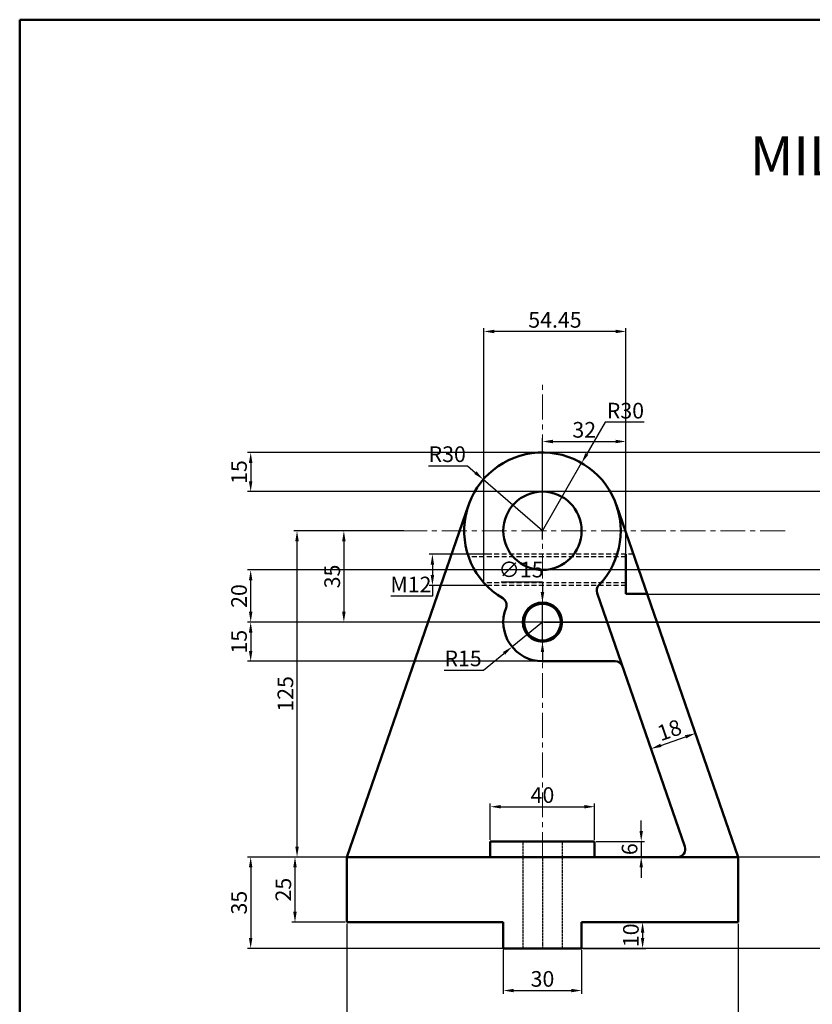
# Model space of a CAD drawing. Units: millimetres. Extents: x 177 to 1064, y 105 to 671.
# Tile 2 of 4: x 177 to 480, y 294 to 671. Entities that reach past the tile are written whole.
import ezdxf

# ---------------------------------------------------------------- set-up
doc = ezdxf.new("R2010")
doc.units = ezdxf.units.MM
doc.header["$LTSCALE"] = 0.3
doc.linetypes.add('CENTER', pattern=[50.8, 31.75, -6.35, 6.35, -6.35])
doc.linetypes.add('HIDDEN', pattern=[9.525, 6.35, -3.175])
for name, color, linetype, lineweight in [('M-CNTR', 1, 'CENTER', 18), ('M-DIMS', 2, 'Continuous', 25), ('M-HIDN', 6, 'HIDDEN', 25), ('M-OUTL', 7, 'Continuous', 50), ('M-TEXT', 3, 'Continuous', 25)]:
    doc.layers.add(name, color=color, linetype=linetype, lineweight=lineweight)
doc.styles.get("Standard").update_dxf_attribs({"font": 'arial.ttf'})
doc.dimstyles.new('ISO-25', dxfattribs={"dimtxt": 6, "dimasz": 4, "dimexe": 1.25, "dimexo": 0.625, "dimtad": 1, "dimtoh": 1, "dimtxsty": 'Standard', "dimcen": 2.5, "dimadec": 0, "dimazin": 0, "dimtfac": 1, "dimtmove": 0, "dimatfit": 3, "dimfxl": 1, "dimarcsym": 0})

# ---------------------------------------------------------------- blocks, each defined once
blk = doc.blocks.new('*D1')
at = {"layer": 'Defpoints', "color": 0, "ltscale": 0.2, "transparency": 16777216}
for p in [(302.04, 325.34), (452.04, 325.34), (452.04, 278.47)]:
    blk.add_point(p, dxfattribs=at)
at = {"layer": 'M-DIMS', "color": 0, "lineweight": -2, "ltscale": 0.2, "transparency": 16777216}
for p, q in [((302.04, 324.72), (302.04, 277.22)), ((452.04, 324.72), (452.04, 277.22)), ((306.04, 278.47), (448.04, 278.47))]:
    blk.add_line(p, q, dxfattribs=at)
at = {"layer": 'M-DIMS', "color": 0, "ltscale": 0.2, "transparency": 16777216}
for points in [[(306.04, 279.14), (306.04, 277.81), (302.04, 278.47)], [(448.04, 279.14), (448.04, 277.81), (452.04, 278.47)]]:
    blk.add_solid(points, dxfattribs=at)
at = {"layer": 'M-DIMS', "color": 0, "ltscale": 0.2, "transparency": 16777216, "insert": (377.04, 282.16), "char_height": 6, "attachment_point": 5}
blk.add_mtext('150', dxfattribs=at)
blk = doc.blocks.new('*D2')
at = {"layer": 'Defpoints', "color": 0, "ltscale": 0.2, "transparency": 16777216}
for p in [(362.04, 315.34), (392.04, 315.34), (392.04, 299.16)]:
    blk.add_point(p, dxfattribs=at)
at = {"layer": 'M-DIMS', "color": 0, "lineweight": -2, "ltscale": 0.2, "transparency": 16777216}
for p, q in [((362.04, 314.72), (362.04, 297.91)), ((392.04, 314.72), (392.04, 297.91)), ((366.04, 299.16), (388.04, 299.16))]:
    blk.add_line(p, q, dxfattribs=at)
at = {"layer": 'M-DIMS', "color": 0, "ltscale": 0.2, "transparency": 16777216}
for points in [[(366.04, 299.83), (366.04, 298.5), (362.04, 299.16)], [(388.04, 299.83), (388.04, 298.5), (392.04, 299.16)]]:
    blk.add_solid(points, dxfattribs=at)
at = {"layer": 'M-DIMS', "color": 0, "ltscale": 0.2, "transparency": 16777216, "insert": (377.04, 302.85), "char_height": 6, "attachment_point": 5}
blk.add_mtext('30', dxfattribs=at)
blk = doc.blocks.new('*D3')
at = {"layer": 'Defpoints', "color": 0, "ltscale": 0.2, "transparency": 16777216}
for p in [(302.04, 350.34), (282.23, 325.34), (302.04, 325.34)]:
    blk.add_point(p, dxfattribs=at)
at = {"layer": 'M-DIMS', "color": 0, "lineweight": -2, "ltscale": 0.2, "transparency": 16777216}
for p, q in [((301.42, 350.34), (280.98, 350.34)), ((282.23, 346.34), (282.23, 329.34)), ((301.42, 325.34), (280.98, 325.34))]:
    blk.add_line(p, q, dxfattribs=at)
at = {"layer": 'M-DIMS', "color": 0, "ltscale": 0.2, "transparency": 16777216}
for points in [[(281.56, 346.34), (282.89, 346.34), (282.23, 350.34)], [(281.56, 329.34), (282.89, 329.34), (282.23, 325.34)]]:
    blk.add_solid(points, dxfattribs=at)
at = {"layer": 'M-DIMS', "color": 0, "ltscale": 0.2, "transparency": 16777216, "insert": (278.54, 337.84), "char_height": 6, "attachment_point": 5, "rotation": 90}
blk.add_mtext('25', dxfattribs=at)
blk = doc.blocks.new('*D4')
at = {"layer": 'Defpoints', "color": 0, "ltscale": 0.2, "transparency": 16777216}
for p in [(283.01, 475.34), (302.04, 475.34), (302.04, 350.34)]:
    blk.add_point(p, dxfattribs=at)
at = {"layer": 'M-DIMS', "color": 0, "lineweight": -2, "ltscale": 0.2, "transparency": 16777216}
for p, q in [((301.42, 475.34), (281.76, 475.34)), ((283.01, 354.34), (283.01, 471.34)), ((301.42, 350.34), (281.76, 350.34))]:
    blk.add_line(p, q, dxfattribs=at)
at = {"layer": 'M-DIMS', "color": 0, "ltscale": 0.2, "transparency": 16777216}
for points in [[(282.35, 471.34), (283.68, 471.34), (283.01, 475.34)], [(282.35, 354.34), (283.68, 354.34), (283.01, 350.34)]]:
    blk.add_solid(points, dxfattribs=at)
at = {"layer": 'M-DIMS', "color": 0, "ltscale": 0.2, "transparency": 16777216, "insert": (279.33, 412.84), "char_height": 6, "attachment_point": 5, "rotation": 90}
blk.add_mtext('125', dxfattribs=at)
blk = doc.blocks.new('*D5')
at = {"layer": 'Defpoints', "color": 0, "ltscale": 0.2, "transparency": 16777216}
for p in [(397.04, 369.61), (357.04, 356.34), (397.04, 356.34)]:
    blk.add_point(p, dxfattribs=at)
at = {"layer": 'M-DIMS', "color": 0, "lineweight": -2, "ltscale": 0.2, "transparency": 16777216}
for p, q in [((357.04, 356.97), (357.04, 370.86)), ((397.04, 356.97), (397.04, 370.86)), ((361.04, 369.61), (393.04, 369.61))]:
    blk.add_line(p, q, dxfattribs=at)
at = {"layer": 'M-DIMS', "color": 0, "ltscale": 0.2, "transparency": 16777216}
for points in [[(361.04, 370.28), (361.04, 368.94), (357.04, 369.61)], [(393.04, 370.28), (393.04, 368.94), (397.04, 369.61)]]:
    blk.add_solid(points, dxfattribs=at)
at = {"layer": 'M-DIMS', "color": 0, "ltscale": 0.2, "transparency": 16777216, "insert": (377.04, 373.3), "char_height": 6, "attachment_point": 5}
blk.add_mtext('40', dxfattribs=at)
blk = doc.blocks.new('*D6')
at = {"layer": 'Defpoints', "color": 0, "ltscale": 0.2, "transparency": 16777216}
for p in [(397.04, 356.34), (397.04, 350.34), (414.87, 350.34)]:
    blk.add_point(p, dxfattribs=at)
at = {"layer": 'M-DIMS', "color": 0, "lineweight": -2, "ltscale": 0.2, "transparency": 16777216}
for p, q in [((414.87, 360.34), (414.87, 364.34)), ((397.67, 356.34), (416.12, 356.34)), ((414.87, 356.34), (414.87, 350.34)), ((397.67, 350.34), (416.12, 350.34)), ((414.87, 346.34), (414.87, 342.34))]:
    blk.add_line(p, q, dxfattribs=at)
at = {"layer": 'M-DIMS', "color": 0, "ltscale": 0.2, "transparency": 16777216}
for points in [[(414.21, 360.34), (415.54, 360.34), (414.87, 356.34)], [(414.21, 346.34), (415.54, 346.34), (414.87, 350.34)]]:
    blk.add_solid(points, dxfattribs=at)
at = {"layer": 'M-DIMS', "color": 0, "ltscale": 0.2, "transparency": 16777216, "insert": (411.19, 353.34), "char_height": 6, "attachment_point": 5, "rotation": 90}
blk.add_mtext('6', dxfattribs=at)
blk = doc.blocks.new('*D7')
at = {"layer": 'Defpoints', "color": 0, "ltscale": 0.2, "transparency": 16777216}
for p in [(392.04, 325.34), (392.04, 315.34), (415.4, 315.34)]:
    blk.add_point(p, dxfattribs=at)
at = {"layer": 'M-DIMS', "color": 0, "lineweight": -2, "ltscale": 0.2, "transparency": 16777216}
for p, q in [((392.67, 325.34), (416.65, 325.34)), ((415.4, 321.34), (415.4, 319.34)), ((392.67, 315.34), (416.65, 315.34))]:
    blk.add_line(p, q, dxfattribs=at)
at = {"layer": 'M-DIMS', "color": 0, "ltscale": 0.2, "transparency": 16777216}
for points in [[(414.74, 321.34), (416.07, 321.34), (415.4, 325.34)], [(414.74, 319.34), (416.07, 319.34), (415.4, 315.34)]]:
    blk.add_solid(points, dxfattribs=at)
at = {"layer": 'M-DIMS', "color": 0, "ltscale": 0.2, "transparency": 16777216, "insert": (411.71, 320.34), "char_height": 6, "attachment_point": 5, "rotation": 90}
blk.add_mtext('10', dxfattribs=at)
blk = doc.blocks.new('*D8')
at = {"layer": 'Defpoints', "color": 0, "ltscale": 0.2, "transparency": 16777216}
for p in [(324.6, 475.34), (300.95, 440.34), (324.6, 440.34)]:
    blk.add_point(p, dxfattribs=at)
at = {"layer": 'M-DIMS', "color": 0, "lineweight": -2, "ltscale": 0.2, "transparency": 16777216}
for p, q in [((323.98, 475.34), (299.7, 475.34)), ((300.95, 471.34), (300.95, 444.34)), ((323.98, 440.34), (299.7, 440.34))]:
    blk.add_line(p, q, dxfattribs=at)
at = {"layer": 'M-DIMS', "color": 0, "ltscale": 0.2, "transparency": 16777216}
for points in [[(300.29, 471.34), (301.62, 471.34), (300.95, 475.34)], [(300.29, 444.34), (301.62, 444.34), (300.95, 440.34)]]:
    blk.add_solid(points, dxfattribs=at)
at = {"layer": 'M-DIMS', "color": 0, "ltscale": 0.2, "transparency": 16777216, "insert": (297.26, 457.84), "char_height": 6, "attachment_point": 5, "rotation": 90}
blk.add_mtext('35', dxfattribs=at)
blk = doc.blocks.new('*D9')
at = {"layer": 'Defpoints', "color": 0, "ltscale": 0.2, "transparency": 16777216}
for p in [(358.09, 466.34), (334.88, 454.34), (358.09, 454.34)]:
    blk.add_point(p, dxfattribs=at)
at = {"layer": 'M-DIMS', "color": 0, "lineweight": -2, "ltscale": 0.2, "transparency": 16777216}
for p, q in [((357.46, 466.34), (333.63, 466.34)), ((334.88, 462.34), (334.88, 458.34)), ((357.46, 454.34), (333.63, 454.34)), ((334.88, 454.34), (334.88, 450.34)), ((334.88, 450.34), (319.01, 450.34))]:
    blk.add_line(p, q, dxfattribs=at)
at = {"layer": 'M-DIMS', "color": 0, "ltscale": 0.2, "transparency": 16777216}
for points in [[(334.21, 462.34), (335.54, 462.34), (334.88, 466.34)], [(334.21, 458.34), (335.54, 458.34), (334.88, 454.34)]]:
    blk.add_solid(points, dxfattribs=at)
at = {"layer": 'M-DIMS', "color": 0, "ltscale": 0.2, "transparency": 16777216, "insert": (326.63, 453.98), "char_height": 6, "attachment_point": 5}
blk.add_mtext('M12', dxfattribs=at)
blk = doc.blocks.new('*D10')
at = {"layer": 'Defpoints', "color": 0, "ltscale": 0.2, "transparency": 16777216}
for p in [(409.04, 509.56), (377.04, 471.33), (409.04, 462.03)]:
    blk.add_point(p, dxfattribs=at)
at = {"layer": 'M-DIMS', "color": 0, "lineweight": -2, "ltscale": 0.2, "transparency": 16777216}
for p, q in [((377.04, 471.95), (377.04, 510.81)), ((381.04, 509.56), (405.04, 509.56)), ((409.04, 462.65), (409.04, 510.81))]:
    blk.add_line(p, q, dxfattribs=at)
at = {"layer": 'M-DIMS', "color": 0, "ltscale": 0.2, "transparency": 16777216}
for points in [[(381.04, 510.22), (381.04, 508.89), (377.04, 509.56)], [(405.04, 510.22), (405.04, 508.89), (409.04, 509.56)]]:
    blk.add_solid(points, dxfattribs=at)
at = {"layer": 'M-DIMS', "color": 0, "ltscale": 0.2, "transparency": 16777216, "insert": (393.04, 513.25), "char_height": 6, "attachment_point": 5}
blk.add_mtext('32', dxfattribs=at)
blk = doc.blocks.new('*D11')
at = {"layer": 'Defpoints', "color": 0, "ltscale": 0.2, "transparency": 16777216}
for p in [(435.65, 397.71), (435.65, 397.71), (418.64, 391.82)]:
    blk.add_point(p, dxfattribs=at)
at = {"layer": 'M-DIMS', "color": 0, "lineweight": -2, "ltscale": 0.2, "transparency": 16777216}
for p, q in [((422.42, 393.13), (431.87, 396.4)), ((435.45, 398.3), (435.24, 398.89)), ((418.44, 392.41), (418.23, 393))]:
    blk.add_line(p, q, dxfattribs=at)
at = {"layer": 'M-DIMS', "color": 0, "ltscale": 0.2, "transparency": 16777216}
for points in [[(431.65, 397.03), (432.09, 395.77), (435.65, 397.71)], [(422.2, 393.76), (422.64, 392.5), (418.64, 391.82)]]:
    blk.add_solid(points, dxfattribs=at)
at = {"layer": 'M-DIMS', "color": 0, "ltscale": 0.2, "transparency": 16777216, "insert": (425.94, 398.25), "char_height": 6, "attachment_point": 5, "rotation": 19.0875}
blk.add_mtext('18', dxfattribs=at)
blk = doc.blocks.new('*D12')
at = {"layer": 'Defpoints', "color": 0, "ltscale": 0.2, "transparency": 16777216}
for p in [(377.04, 440.34), (365.4, 430.89)]:
    blk.add_point(p, dxfattribs=at)
at = {"layer": 'M-DIMS', "color": 0, "lineweight": -2, "ltscale": 0.2, "transparency": 16777216}
for p, q in [((377.04, 440.34), (365.4, 430.89)), ((354.43, 421.98), (362.3, 428.36)), ((339.43, 421.98), (354.43, 421.98))]:
    blk.add_line(p, q, dxfattribs=at)
at = {"layer": 'M-DIMS', "color": 0, "ltscale": 0.2, "transparency": 16777216}
blk.add_solid([(361.87, 428.88), (362.72, 427.85), (365.4, 430.89)], dxfattribs=at)
at = {"layer": 'M-DIMS', "color": 0, "ltscale": 0.2, "transparency": 16777216, "insert": (346.62, 425.67), "char_height": 6, "attachment_point": 5}
blk.add_mtext('R15', dxfattribs=at)
blk = doc.blocks.new('*D13')
at = {"layer": 'Defpoints', "color": 0, "ltscale": 0.2, "transparency": 16777216}
for p in [(354.37, 494.99), (377.04, 475.34)]:
    blk.add_point(p, dxfattribs=at)
at = {"layer": 'M-DIMS', "color": 0, "lineweight": -2, "ltscale": 0.2, "transparency": 16777216}
for p, q in [((333.39, 500.23), (348.33, 500.23)), ((348.33, 500.23), (351.35, 497.61)), ((377.04, 475.34), (354.37, 494.99))]:
    blk.add_line(p, q, dxfattribs=at)
at = {"layer": 'M-DIMS', "color": 0, "ltscale": 0.2, "transparency": 16777216}
blk.add_solid([(351.79, 498.12), (350.92, 497.11), (354.37, 494.99)], dxfattribs=at)
at = {"layer": 'M-DIMS', "color": 0, "ltscale": 0.2, "transparency": 16777216, "insert": (340.55, 503.92), "char_height": 6, "attachment_point": 5}
blk.add_mtext('R30', dxfattribs=at)
blk = doc.blocks.new('*D50')
at = {"layer": 'Defpoints', "color": 0, "ltscale": 0.3, "transparency": 16777216}
for p in [(377.04, 440.34), (265.25, 425.34), (377.04, 425.34)]:
    blk.add_point(p, dxfattribs=at)
at = {"layer": 'M-DIMS', "color": 0, "lineweight": -2, "ltscale": 0.3, "transparency": 16777216}
for p, q in [((376.42, 440.34), (264, 440.34)), ((265.25, 436.34), (265.25, 429.34)), ((376.42, 425.34), (264, 425.34))]:
    blk.add_line(p, q, dxfattribs=at)
at = {"layer": 'M-DIMS', "color": 0, "ltscale": 0.3, "transparency": 16777216}
for points in [[(264.58, 436.34), (265.92, 436.34), (265.25, 440.34)], [(264.58, 429.34), (265.92, 429.34), (265.25, 425.34)]]:
    blk.add_solid(points, dxfattribs=at)
at = {"layer": 'M-DIMS', "color": 0, "ltscale": 0.3, "transparency": 16777216, "insert": (261.56, 432.84), "char_height": 6, "attachment_point": 5, "rotation": 90}
blk.add_mtext('15', dxfattribs=at)
blk = doc.blocks.new('*D51')
at = {"layer": 'Defpoints', "color": 0, "ltscale": 0.3, "transparency": 16777216}
for p in [(409.04, 451.12), (377.04, 440.34), (670.3, 440.34)]:
    blk.add_point(p, dxfattribs=at)
at = {"layer": 'M-DIMS', "color": 0, "lineweight": -2, "ltscale": 0.3, "transparency": 16777216}
for p, q in [((409.67, 451.12), (671.55, 451.12)), ((670.3, 447.12), (670.3, 444.34)), ((377.67, 440.34), (671.55, 440.34)), ((670.3, 440.34), (670.3, 436.34)), ((670.3, 436.34), (646.49, 436.34))]:
    blk.add_line(p, q, dxfattribs=at)
at = {"layer": 'M-DIMS', "color": 0, "ltscale": 0.3, "transparency": 16777216}
for points in [[(669.63, 447.12), (670.96, 447.12), (670.3, 451.12)], [(669.63, 444.34), (670.96, 444.34), (670.3, 440.34)]]:
    blk.add_solid(points, dxfattribs=at)
at = {"layer": 'M-DIMS', "color": 0, "ltscale": 0.3, "transparency": 16777216, "insert": (658.08, 440.03), "char_height": 6, "attachment_point": 5}
blk.add_mtext('10.781', dxfattribs=at)
blk = doc.blocks.new('*D52')
at = {"layer": 'Defpoints', "color": 0, "ltscale": 0.3, "transparency": 16777216}
for p in [(354.6, 551.72), (354.6, 455.43), (409.04, 455.34)]:
    blk.add_point(p, dxfattribs=at)
at = {"layer": 'M-DIMS', "color": 0, "lineweight": -2, "ltscale": 0.3, "transparency": 16777216}
for p, q in [((354.6, 456.06), (354.6, 552.97)), ((405.04, 551.72), (358.6, 551.72)), ((409.04, 455.97), (409.04, 552.97))]:
    blk.add_line(p, q, dxfattribs=at)
at = {"layer": 'M-DIMS', "color": 0, "ltscale": 0.3, "transparency": 16777216}
for points in [[(358.6, 552.39), (358.6, 551.05), (354.6, 551.72)], [(405.04, 552.39), (405.04, 551.05), (409.04, 551.72)]]:
    blk.add_solid(points, dxfattribs=at)
at = {"layer": 'M-DIMS', "color": 0, "ltscale": 0.3, "transparency": 16777216, "insert": (381.82, 555.39), "char_height": 6, "attachment_point": 5}
blk.add_mtext('54.45', dxfattribs=at)
blk = doc.blocks.new('*D54')
at = {"layer": 'Defpoints', "color": 0, "ltscale": 0.3, "transparency": 16777216}
for p in [(500.2, 505.34), (265.25, 490.34), (500.2, 490.34)]:
    blk.add_point(p, dxfattribs=at)
at = {"layer": 'M-DIMS', "color": 0, "lineweight": -2, "ltscale": 0.3, "transparency": 16777216}
for p, q in [((499.57, 505.34), (264, 505.34)), ((265.25, 501.34), (265.25, 494.34)), ((499.57, 490.34), (264, 490.34))]:
    blk.add_line(p, q, dxfattribs=at)
at = {"layer": 'M-DIMS', "color": 0, "ltscale": 0.3, "transparency": 16777216}
for points in [[(264.58, 501.34), (265.92, 501.34), (265.25, 505.34)], [(264.58, 494.34), (265.92, 494.34), (265.25, 490.34)]]:
    blk.add_solid(points, dxfattribs=at)
at = {"layer": 'M-DIMS', "color": 0, "ltscale": 0.3, "transparency": 16777216, "insert": (261.56, 497.84), "char_height": 6, "attachment_point": 5, "rotation": 90}
blk.add_mtext('15', dxfattribs=at)
blk = doc.blocks.new('*D55')
at = {"layer": 'Defpoints', "color": 0, "ltscale": 0.3, "transparency": 16777216}
for p in [(265.25, 460.34), (500.2, 460.34), (527.44, 440.34)]:
    blk.add_point(p, dxfattribs=at)
at = {"layer": 'M-DIMS', "color": 0, "lineweight": -2, "ltscale": 0.3, "transparency": 16777216}
for p, q in [((499.57, 460.34), (264, 460.34)), ((265.25, 444.34), (265.25, 456.34)), ((526.82, 440.34), (264, 440.34))]:
    blk.add_line(p, q, dxfattribs=at)
at = {"layer": 'M-DIMS', "color": 0, "ltscale": 0.3, "transparency": 16777216}
for points in [[(264.58, 456.34), (265.92, 456.34), (265.25, 460.34)], [(264.58, 444.34), (265.92, 444.34), (265.25, 440.34)]]:
    blk.add_solid(points, dxfattribs=at)
at = {"layer": 'M-DIMS', "color": 0, "ltscale": 0.3, "transparency": 16777216, "insert": (261.56, 450.34), "char_height": 6, "attachment_point": 5, "rotation": 90}
blk.add_mtext('20', dxfattribs=at)
blk = doc.blocks.new('*D57')
at = {"layer": 'Defpoints', "color": 0, "ltscale": 0.3, "transparency": 16777216}
for p in [(521.2, 350.34), (265.25, 315.34), (500.2, 315.34)]:
    blk.add_point(p, dxfattribs=at)
at = {"layer": 'M-DIMS', "color": 0, "lineweight": -2, "ltscale": 0.3, "transparency": 16777216}
for p, q in [((520.57, 350.34), (264, 350.34)), ((265.25, 346.34), (265.25, 319.34)), ((499.57, 315.34), (264, 315.34))]:
    blk.add_line(p, q, dxfattribs=at)
at = {"layer": 'M-DIMS', "color": 0, "ltscale": 0.3, "transparency": 16777216}
for points in [[(264.58, 346.34), (265.92, 346.34), (265.25, 350.34)], [(264.58, 319.34), (265.92, 319.34), (265.25, 315.34)]]:
    blk.add_solid(points, dxfattribs=at)
at = {"layer": 'M-DIMS', "color": 0, "ltscale": 0.3, "transparency": 16777216, "insert": (261.56, 332.84), "char_height": 6, "attachment_point": 5, "rotation": 90}
blk.add_mtext('35', dxfattribs=at)
blk = doc.blocks.new('*D68')
at = {"layer": 'Defpoints', "color": 0, "ltscale": 0.3, "transparency": 16777216}
for p in [(392.04, 501.32), (377.04, 475.34)]:
    blk.add_point(p, dxfattribs=at)
at = {"layer": 'M-DIMS', "color": 0, "lineweight": -2, "ltscale": 0.3, "transparency": 16777216}
for p, q in [((401.04, 516.91), (394.04, 504.79)), ((415.98, 516.91), (401.04, 516.91)), ((377.04, 475.34), (392.04, 501.32))]:
    blk.add_line(p, q, dxfattribs=at)
at = {"layer": 'M-DIMS', "color": 0, "ltscale": 0.3, "transparency": 16777216}
blk.add_solid([(393.46, 505.12), (394.62, 504.45), (392.04, 501.32)], dxfattribs=at)
at = {"layer": 'M-DIMS', "color": 0, "ltscale": 0.3, "transparency": 16777216, "insert": (408.82, 520.6), "char_height": 6, "attachment_point": 5}
blk.add_mtext('R30', dxfattribs=at)
blk = doc.blocks.new('*D69')
at = {"layer": 'Defpoints', "color": 0, "ltscale": 0.3, "transparency": 16777216}
for p in [(377.04, 447.84), (377.05, 432.84)]:
    blk.add_point(p, dxfattribs=at)
at = {"layer": 'M-DIMS', "color": 0, "lineweight": -2, "ltscale": 0.3, "transparency": 16777216}
for p, q in [((361.24, 455.84), (377.04, 455.84)), ((377.04, 455.84), (377.04, 451.84)), ((377.05, 432.84), (377.04, 447.84)), ((377.05, 428.84), (377.05, 424.84))]:
    blk.add_line(p, q, dxfattribs=at)
at = {"layer": 'M-DIMS', "color": 0, "ltscale": 0.3, "transparency": 16777216}
for points in [[(377.7, 451.84), (376.37, 451.84), (377.04, 447.84)], [(377.71, 428.84), (376.38, 428.84), (377.05, 432.84)]]:
    blk.add_solid(points, dxfattribs=at)
at = {"layer": 'M-DIMS', "color": 0, "ltscale": 0.3, "transparency": 16777216, "insert": (368.83, 459.7), "char_height": 6, "attachment_point": 5}
blk.add_mtext('∅15', dxfattribs=at)

msp = doc.modelspace()

# ---------------------------------------------------------------- linework, layer by layer
at = {"layer": 'M-CNTR'}
for p, q in [((377.0432, 350.3423), (377.0432, 531.6184)), ((469.9709, 475.3423), (285.3513, 475.3423)), ((478.9765, 440.3423), (285.3513, 440.3423))]:
    msp.add_line(p, q, dxfattribs=at)
at = {"layer": 'M-HIDN'}
for p, q in [((411.9028, 466.3423), (348.425, 466.3423)), ((409.0432, 465.3423), (348.7589, 465.3423)), ((409.0432, 455.3423), (354.6825, 455.3423)), ((409.0432, 454.3423), (355.6189, 454.3423))]:
    msp.add_line(p, q, dxfattribs=at)
at = {"layer": 'M-HIDN', "ltscale": 0.2}
for p, q in [((369.5432, 356.3423), (369.5432, 315.3423)), ((384.5432, 356.3423), (384.5432, 315.3423)), ((377.0432, 350.3423), (377.0432, 315.3423))]:
    msp.add_line(p, q, dxfattribs=at)
at = {"layer": 'M-OUTL'}
for p, q in [((348.6926, 485.1527), (302.0432, 350.3423)), ((405.3938, 485.1527), (452.0432, 350.3423)), ((409.0432, 451.1235), (409.0432, 466.3423)), ((397.9956, 451.4887), (431.6184, 354.3234)), ((409.0432, 451.1235), (417.1691, 451.1235)), ((377.0432, 425.3423), (404.9067, 425.3423)), ((357.0432, 350.3423), (357.0432, 356.3423)), ((397.0432, 356.3423), (357.0432, 356.3423)), ((397.0432, 350.3423), (397.0432, 356.3423)), ((452.0432, 350.3423), (302.0432, 350.3423)), ((302.0432, 350.3423), (302.0432, 325.3423)), ((452.0432, 325.3423), (452.0432, 350.3423)), ((302.0432, 325.3423), (362.0432, 325.3423)), ((362.0432, 325.3423), (362.0432, 315.3423)), ((392.0432, 315.3423), (392.0432, 325.3423)), ((392.0432, 325.3423), (452.0432, 325.3423)), ((362.0432, 315.3423), (392.0432, 315.3423))]:
    msp.add_line(p, q, dxfattribs=at)
at = {"layer": 'M-OUTL', "ltscale": 0.3}
msp.add_lwpolyline([(176.7558, 671.1865), (1063.6064, 671.1865), (1063.6064, 105.1095), (176.7558, 105.1095)], close=True, dxfattribs=at)
at = {"layer": 'M-OUTL'}
for centre, radius in [((377.0432, 475.3423), 15), ((377.0432, 440.3423), 7.5), ((377.0432, 440.3423), 7)]:
    msp.add_circle(centre, radius, dxfattribs=at)
for centre, radius, start, end in [((377.0432, 475.3423), 30, 316.123213, 239.482247), ((400.8306, 452.4697), 3, 136.123213, 199.087522), ((360.2856, 446.9138), 3, 338.587533, 59.482247), ((377.0432, 440.3423), 15, 158.587533, 270), ((404.9067, 422.3423), 3, 19.087522, 90), ((428.7833, 353.3423), 3, 270, 19.087522)]:
    msp.add_arc(centre, radius, start, end, dxfattribs=at)

# ---------------------------------------------------------------- texts
at = {"layer": 'M-TEXT', "ltscale": 0.3, "insert": (437.8929, 626.4883), "char_height": 15, "attachment_point": 1}
msp.add_mtext_dynamic_manual_height_columns('\\pxqc;MILLING MACHINE TAIL STOCK', width=257.833122, gutter_width=12.5, heights=[0], dxfattribs=at)

# ---------------------------------------------------------------- dimensions: what is measured, and where the dimension line sits
at = {"layer": 'M-DIMS', "ltscale": 0.3}
dim = msp.add_linear_dim(base=(354.5977, 551.7184), p1=(409.0432, 455.3423), p2=(354.5977, 455.4348), dimstyle='ISO-25', override={"dimdec": 2, "dimlfac": 1, "dimrnd": 0, "dimzin": 0, "dimdsep": 46, "dimlunit": 2}, dxfattribs=at)
dim.commit()
dim.dimension.update_dxf_attribs({"geometry": '*D52', "text_midpoint": (381.8204, 555.3946)})
dim = msp.add_radius_dim(center=(377.0432, 475.3423), mpoint=(392.0421, 501.3237), dimstyle='ISO-25', override={"dimdec": 0, "dimlfac": 1, "dimrnd": 0, "dimzin": 0, "dimdsep": 46, "dimlunit": 2}, dxfattribs=at)
dim.commit()
dim.dimension.update_dxf_attribs({"geometry": '*D68', "text_midpoint": (408.8248, 516.9125), "dimtype": 164})
at = {"layer": 'M-DIMS', "ltscale": 0.2}
for base, p1, p2, picture, middle in [((409.0432, 509.5571), (377.0432, 471.3279), (409.0432, 462.0255), '*D10', (393.0432, 513.2475)), ((397.0432, 369.6096), (357.0432, 356.3423), (397.0432, 356.3423), '*D5', (377.0432, 373.2981)), ((452.0432, 278.4731), (302.0432, 325.3423), (452.0432, 325.3423), '*D1', (377.0432, 282.1615)), ((392.0432, 299.1617), (362.0432, 315.3423), (392.0432, 315.3423), '*D2', (377.0432, 302.8522))]:
    dim = msp.add_linear_dim(base=base, p1=p1, p2=p2, dimstyle='ISO-25', override={"dimclrd": 0, "dimclre": 0, "dimclrt": 0}, dxfattribs=at)
    dim.commit()
    dim.dimension.update_dxf_attribs({"geometry": picture, "text_midpoint": middle})
for center, mpoint, picture, middle in [((377.0432, 475.3423), (354.3749, 494.9931), '*D13', (340.5468, 503.9238)), ((377.0432, 440.3423), (365.4, 430.8852), '*D12', (346.6186, 425.6671))]:
    dim = msp.add_radius_dim(center=center, mpoint=mpoint, dimstyle='ISO-25', override={"dimclrd": 0, "dimclre": 0, "dimclrt": 0}, dxfattribs=at)
    dim.commit()
    dim.dimension.update_dxf_attribs({"geometry": picture, "text_midpoint": middle})
at = {"layer": 'M-DIMS', "ltscale": 0.3}
for base, p1, p2, override, picture, middle in [((265.2513, 490.3423), (500.1968, 505.3423), (500.1968, 490.3423), {"dimdec": 0, "dimlfac": 1, "dimrnd": 0, "dimzin": 0, "dimdsep": 46, "dimlunit": 2}, '*D54', (261.5629, 497.8423)), ((265.2513, 460.3423), (527.444, 440.3423), (500.1968, 460.3423), {"dimdec": 0, "dimlfac": 1, "dimrnd": 0, "dimzin": 0, "dimdsep": 46, "dimlunit": 2}, '*D55', (261.5629, 450.3423)), ((670.2968, 440.3423), (409.0432, 451.1235), (377.0432, 440.3423), {"dimdec": 3, "dimlfac": 1, "dimrnd": 0, "dimzin": 0, "dimdsep": 46, "dimlunit": 2}, '*D51', (658.079, 440.0308)), ((265.2513, 425.3423), (377.0432, 440.3423), (377.0432, 425.3423), {"dimdec": 0, "dimlfac": 1, "dimrnd": 0, "dimzin": 0, "dimdsep": 46, "dimlunit": 2}, '*D50', (261.5629, 432.8423)), ((265.2513, 315.3423), (521.1968, 350.3423), (500.1968, 315.3423), {"dimdec": 0, "dimlfac": 1, "dimrnd": 0, "dimzin": 0, "dimdsep": 46, "dimlunit": 2}, '*D57', (261.5608, 332.8423))]:
    dim = msp.add_linear_dim(base=base, p1=p1, p2=p2, angle=90, dimstyle='ISO-25', override=override, dxfattribs=at)
    dim.commit()
    dim.dimension.update_dxf_attribs({"geometry": picture, "text_midpoint": middle})
at = {"layer": 'M-DIMS', "ltscale": 0.2}
for base, p1, p2, picture, middle in [((283.0137, 475.3423), (302.0432, 350.3423), (302.0432, 475.3423), '*D4', (279.3252, 412.8423)), ((300.9541, 440.3423), (324.6048, 475.3423), (324.6048, 440.3423), '*D8', (297.2636, 457.8423)), ((414.8747, 350.3423), (397.0432, 356.3423), (397.0432, 350.3423), '*D6', (411.1863, 353.3423)), ((282.2262, 325.3423), (302.0432, 350.3423), (302.0432, 325.3423), '*D3', (278.5378, 337.8423)), ((415.4026, 315.3423), (392.0432, 325.3423), (392.0432, 315.3423), '*D7', (411.7142, 320.3423))]:
    dim = msp.add_linear_dim(base=base, p1=p1, p2=p2, angle=90, dimstyle='ISO-25', override={"dimclrd": 0, "dimclre": 0, "dimclrt": 0}, dxfattribs=at)
    dim.commit()
    dim.dimension.update_dxf_attribs({"geometry": picture, "text_midpoint": middle})
dim = msp.add_linear_dim(base=(334.8751, 454.3423), p1=(358.0888, 466.3423), p2=(358.0888, 454.3423), angle=90, text='M<>', dimstyle='ISO-25', override={"dimclrd": 0, "dimclre": 0, "dimclrt": 0}, dxfattribs=at)
dim.commit()
dim.dimension.update_dxf_attribs({"geometry": '*D9', "text_midpoint": (326.6293, 453.9796)})
at = {"layer": 'M-DIMS', "ltscale": 0.3}
dim = msp.add_diameter_dim_2p(p1=(377.0463, 432.8423), p2=(377.04, 447.8423), dimstyle='ISO-25', override={"dimdec": 0, "dimlfac": 1, "dimrnd": 0, "dimzin": 0, "dimdsep": 46, "dimlunit": 2}, dxfattribs=at)
dim.commit()
dim.dimension.update_dxf_attribs({"geometry": '*D69', "text_midpoint": (368.8277, 455.8423), "dimtype": 163})
at = {"layer": 'M-DIMS', "ltscale": 0.2}
dim = msp.add_aligned_dim(p1=(418.6423, 391.8223), p2=(435.6527, 397.7086), distance=0, dimstyle='ISO-25', override={"dimclrd": 0, "dimclre": 0, "dimclrt": 0}, dxfattribs=at)
dim.commit()
dim.dimension.update_dxf_attribs({"geometry": '*D11', "text_midpoint": (425.9413, 398.2511)})

doc.saveas('drawing.dxf')
